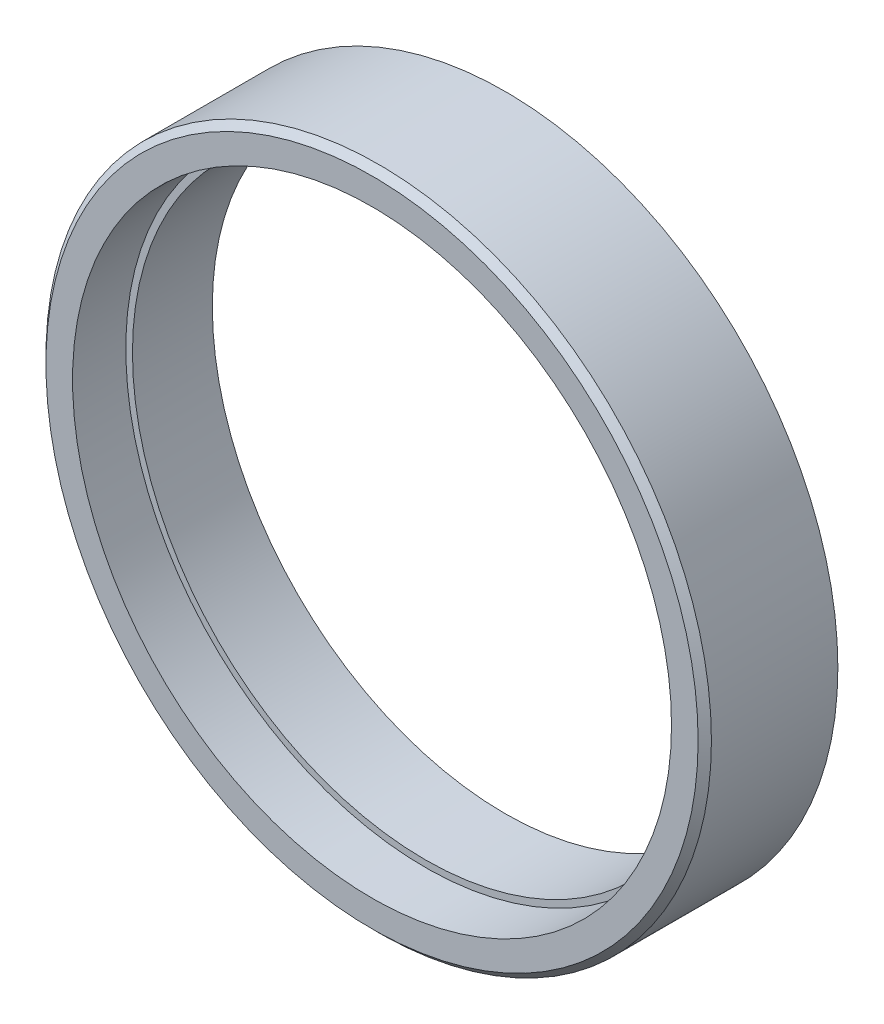
from build123d import *

# Parameters (mm, degrees)
RIM_OD_SKETCH_100_R       = 50
RIM_BLANK_100X20_DEPTH    = 20
RECESS_SKETCH_90_R        = 45
RECESS_90X8_DEPTH         = 8
BORE_SKETCH_88_R          = 44
BORE_88_THROUGH_DEPTH     = 50
EDGE_CHAMFER_1X45DEG_SIZE = 1


with BuildPart() as part:
    # Rim OD Sketch Ø100 → Rim Blank Ø100x20 (new body)
    with BuildSketch(Plane.XY):
        Circle(RIM_OD_SKETCH_100_R)
    extrude(amount=RIM_BLANK_100X20_DEPTH)

    # Recess Sketch Ø90 → Recess Ø90x8 (cut)
    with BuildSketch(Plane.XY.offset(20)):
        Circle(RECESS_SKETCH_90_R)
    extrude(amount=-RECESS_90X8_DEPTH, mode=Mode.SUBTRACT)

    # Bore Sketch Ø88 → Bore Ø88 Through (cut)
    with BuildSketch(Plane.XY.offset(12)):
        Circle(BORE_SKETCH_88_R)
    extrude(amount=-BORE_88_THROUGH_DEPTH, mode=Mode.SUBTRACT)

    # Edge Chamfer 1x45deg
    edge_chamfer_1x45deg_edges = [part.edges().sort_by_distance(p)[0] for p in [
        (-50, 0, 20),
    ]]
    chamfer(edge_chamfer_1x45deg_edges, length=EDGE_CHAMFER_1X45DEG_SIZE)


solid = part.part
